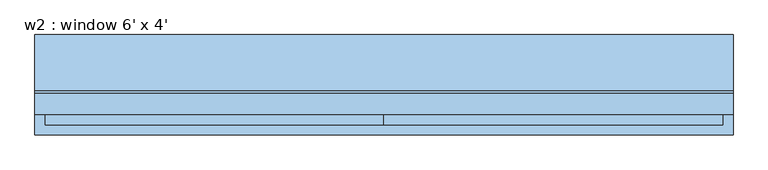
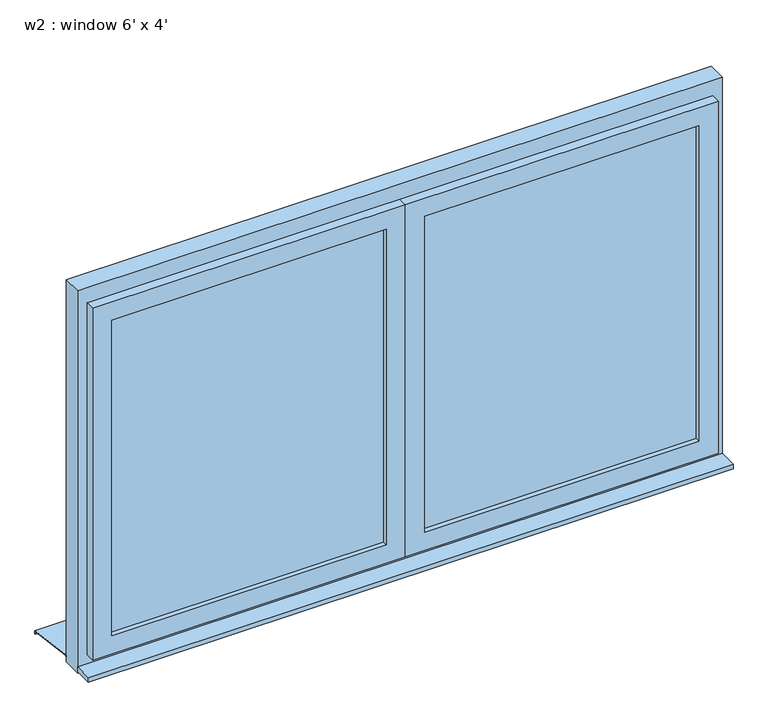
"""IFC4 building model written with IfcOpenShell, lengths in millimetres: window geometry, w2 : window 6' x 4'."""

from ifc_helpers import new_model, si_unit, frame, origin, place, context, project, spatial, polyline, outline, extrude, faceted_brep, source, transform, mapped, element, save


def w2_window_6_x_4_7b90d420(model_context):
    return source(origin(), model_context, "Body", "SolidModel", [
        extrude(outline(polyline([(-15.6778457, 1020.0), (144.3, 1000.0), (144.3, 990.0), (142.3, 990.0), (142.3, 998.3604634), (-15.8759277, 1018.0), (-25.7, 1018.0), (-25.7, 1020.0), (-15.6778457, 1020.0)])), frame((-1005.0, 0.0, 0.0), z_axis=(1.0, 0.0, 0.0), x_axis=(0.0, 1.0, 0.0)), (0.0, 0.0, 1.0), 2010.0),
        extrude(outline(polyline([(-1005.0, -144.3), (-1005.0, -85.7), (1005.0, -85.7), (1005.0, -144.3), (-1005.0, -144.3)])), frame((0.0, 0.0, 1005.0), z_axis=(0.0, 0.0, 1.0), x_axis=(1.0, 0.0, 0.0)), (0.0, 0.0, 1.0), 15.0),
        extrude(outline(polyline([(60.0, -70.7), (915.0, -70.7), (915.0, -100.7), (60.0, -100.7), (60.0, -70.7)])), frame((0.0, 0.0, 1110.0), z_axis=(0.0, 0.0, 1.0), x_axis=(1.0, 0.0, 0.0)), (0.0, 0.0, 1.0), 1040.0),
        extrude(outline(polyline([(-915.0, -70.7), (-60.0, -70.7), (-60.0, -100.7), (-915.0, -100.7), (-915.0, -70.7)])), frame((0.0, 0.0, 1110.0), z_axis=(0.0, 0.0, 1.0), x_axis=(1.0, 0.0, 0.0)), (0.0, 0.0, 1.0), 1040.0),
        extrude(outline(polyline([(2260.0, -1005.0), (1000.0, -1005.0), (1000.0, 1005.0), (2260.0, 1005.0), (2260.0, -1005.0)]), holes=[polyline([(2180.0, -945.0), (2180.0, 945.0), (1080.0, 945.0), (1080.0, -945.0), (2180.0, -945.0)])]), frame((0.0, -85.7, 0.0), z_axis=(0.0, 1.0, 0.0), x_axis=(0.0, 0.0, 1.0)), (0.0, 0.0, 1.0), 60.0),
        extrude(outline(polyline([(30.0, -85.7), (-30.0, -85.7), (-30.0, -25.7), (30.0, -25.7), (30.0, -85.7)])), frame((0.0, 0.0, 1080.0), z_axis=(0.0, 0.0, 1.0), x_axis=(1.0, 0.0, 0.0)), (0.0, 0.0, 1.0), 1100.0),
        faceted_brep([(30.0, -85.7, 1080.0), (30.0, -55.7, 1080.0), (945.0, -55.7, 1080.0), (945.0, -85.7, 1080.0), (945.0, -55.7, 2180.0), (945.0, -85.7, 2180.0), (30.0, -55.7, 2180.0), (915.0, -55.7, 2150.0), (60.0, -55.7, 2150.0), (60.0, -55.7, 1110.0), (915.0, -55.7, 1110.0), (975.0, -85.7, 1050.0), (0.0, -85.7, 1050.0), (0.0, -85.7, 2210.0), (975.0, -85.7, 2210.0), (30.0, -85.7, 2180.0), (0.0, -115.7, 1050.0), (975.0, -115.7, 1050.0), (975.0, -115.7, 2210.0), (0.0, -115.7, 2210.0), (915.0, -115.7, 1110.0), (60.0, -115.7, 1110.0), (60.0, -115.7, 2150.0), (915.0, -115.7, 2150.0)], [[[0, 1, 2, 3]], [[3, 2, 4, 5]], [[2, 1, 6, 4], [7, 8, 9, 10]], [[11, 12, 13, 14], [5, 15, 0, 3]], [[16, 12, 11, 17]], [[17, 11, 14, 18]], [[18, 19, 16, 17], [20, 21, 22, 23]], [[9, 21, 20, 10]], [[10, 20, 23, 7]], [[15, 6, 1, 0]], [[19, 13, 12, 16]], [[8, 22, 21, 9]], [[5, 4, 6, 15]], [[18, 14, 13, 19]], [[7, 23, 22, 8]]]),
        faceted_brep([(-945.0, -85.7, 1080.0), (-945.0, -55.7, 1080.0), (-30.0, -55.7, 1080.0), (-30.0, -85.7, 1080.0), (-30.0, -55.7, 2180.0), (-30.0, -85.7, 2180.0), (-945.0, -55.7, 2180.0), (-60.0, -55.7, 2150.0), (-915.0, -55.7, 2150.0), (-915.0, -55.7, 1110.0), (-60.0, -55.7, 1110.0), (0.0, -85.7, 1050.0), (-975.0, -85.7, 1050.0), (-975.0, -85.7, 2210.0), (0.0, -85.7, 2210.0), (-945.0, -85.7, 2180.0), (-975.0, -115.7, 1050.0), (0.0, -115.7, 1050.0), (0.0, -115.7, 2210.0), (-975.0, -115.7, 2210.0), (-60.0, -115.7, 1110.0), (-915.0, -115.7, 1110.0), (-915.0, -115.7, 2150.0), (-60.0, -115.7, 2150.0)], [[[0, 1, 2, 3]], [[3, 2, 4, 5]], [[2, 1, 6, 4], [7, 8, 9, 10]], [[11, 12, 13, 14], [5, 15, 0, 3]], [[16, 12, 11, 17]], [[17, 11, 14, 18]], [[18, 19, 16, 17], [20, 21, 22, 23]], [[9, 21, 20, 10]], [[10, 20, 23, 7]], [[15, 6, 1, 0]], [[19, 13, 12, 16]], [[8, 22, 21, 9]], [[5, 4, 6, 15]], [[18, 14, 13, 19]], [[7, 23, 22, 8]]]),
    ])


if __name__ == "__main__":
    model = new_model("IFC4")
    model_context = context("Model", 3, world=origin())
    ifc_project = project(units=[si_unit("LENGTHUNIT", "METRE", prefix="MILLI")], contexts=[model_context])
    site = spatial("IfcSite", under=ifc_project)
    building = spatial("IfcBuilding", under=site)
    placement = place(None, origin())
    w2_window_6_x_4_shape = w2_window_6_x_4_7b90d420(model_context)
    element("IfcWindow", 1, ObjectType="w2 : window 6' x 4'", at=placement, inside=building, context=model_context, shape_type="MappedRepresentation", body=[
        mapped(w2_window_6_x_4_shape, transform((0.0, 0.0, 0.0), x_axis=(1.0, 0.0, 0.0), y_axis=(0.0, 1.0, 0.0), z_axis=(0.0, 0.0, 1.0))),
    ])
    save(model, "model.ifc")

# Revit data of these elements
# Type "w2 : window 6' x 4'"
#   Type Mark = "26"
#   Operation = "DoublePanelVertical"
#   Keynote = "16.05.01"
#   Analytic Construction = "<None>"
#   Rough Width = 6' - 7.13386"
#   Rough Height = 4' - 1.6063"
#   Rahmentiefe = 0' - 2.3622"
#   Rahmenhöhe unten = 0' - 3.14961"
#   Rahmehöhe oben = 0' - 3.14961"
#   Rahmenbreite = 0' - 2.3622"
#   Heat Transfer Coefficient (U) = 2.81836 BTU/(h·ft²·°F)
#   Height = 4' - 1.6063"
#   Flügeltiefe = 0' - 2.3622"
#   Flügelbreite = 0' - 2.3622"
#   Einbautiefe (von außen) [instance default] = 0' - 5.51181"
#   Width = 6' - 7.13386"
#   Kippflügel [instance default] = yes
#   Drehflügel im Grundriß darstellen [instance default] = no
#   Drehflügel [instance default] = yes
#   Define Thermal Properties by = 1
#   Rahmen [instance default] = none
#   Glas [instance default] = blue glass
#   Flügel [instance default] = WINDOW COLOUR WHITE
#   Fensterbank aussen [instance default] = WINDOW COLOUR WHITE
#   Fensterbank innen [instance default] = WINDOW COLOUR WHITE
#   Visual Light Transmittance = 0
#   Thermal Resistance (R) = 0
#   Solar Heat Gain Coefficient = 0
#   Wall Closure = (empty or 0)
# Element 1 (IfcWindow, "w2 : window 6' x 4'")
#   Materials on its faces: "WINDOW COLOUR WHITE", "blue glass"
# Materials
#   "blue glass": class "System", colour RGB 0 0 255, transparency 0.75, Cost = 0
#   "WINDOW COLOUR WHITE": class "Generic", colour RGB 120 120 120, transparency 0, Cost = 0
